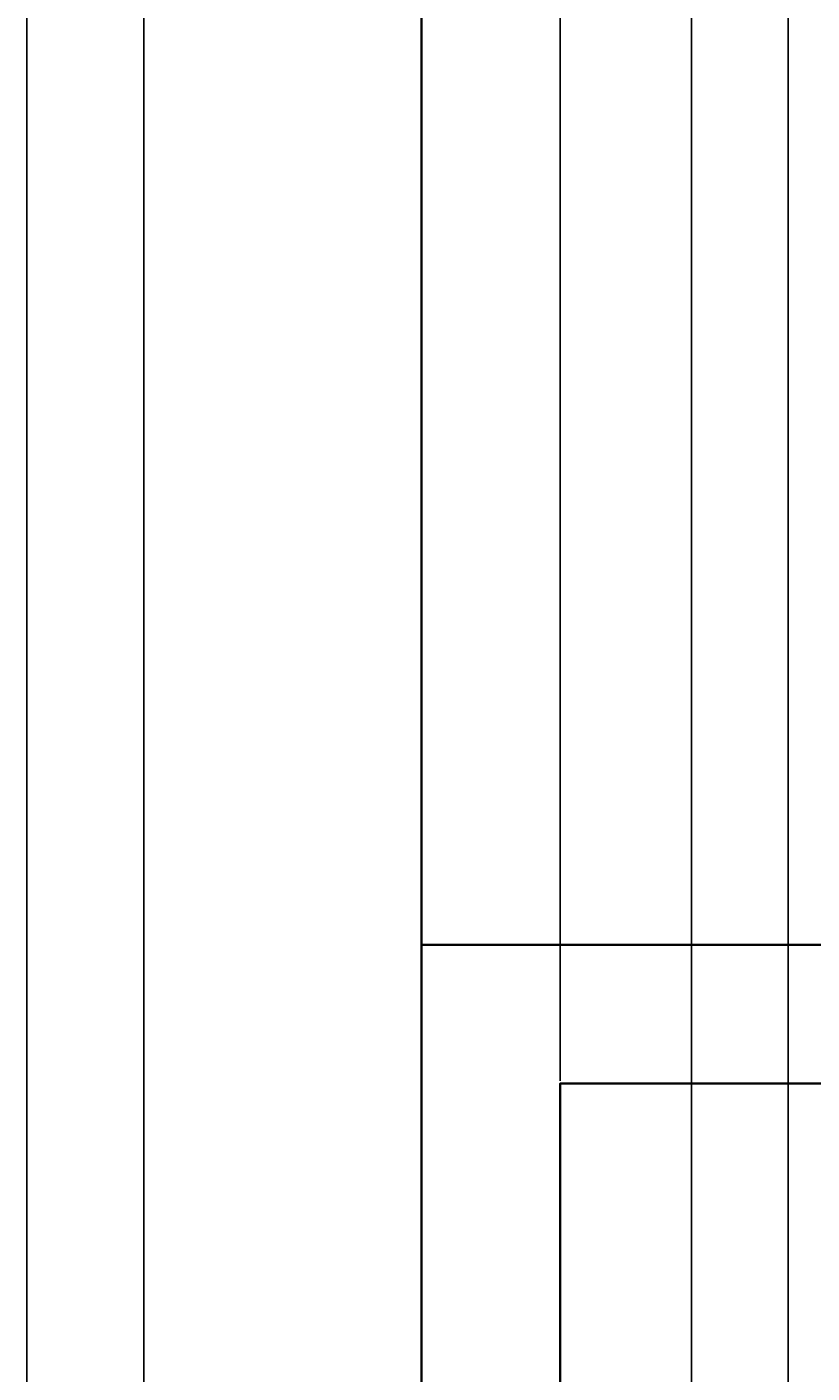
# Model space of a CAD drawing. Units: inches. Extents: x -6 to 289, y -8 to 323.
# Tile 50 of 107: x 107 to 124, y 153 to 182. Entities that reach past the tile are written whole.
import ezdxf

# ---------------------------------------------------------------- set-up
doc = ezdxf.new("R2010")
doc.units = ezdxf.units.IN
doc.header["$MEASUREMENT"] = 0
doc.layers.add('A-ANNO-DIMS', color=2, linetype='Continuous', lineweight=18)
doc.layers.add('A-ELEV', color=7, linetype='Continuous', lineweight=35)
doc.styles.get("Standard").update_dxf_attribs({"font": 'arial.ttf'})
doc.dimstyles.get("Standard").update_dxf_attribs({"dimtxt": 0.18, "dimasz": 0.18, "dimexe": 0.18, "dimexo": 0.0625, "dimgap": 0.09, "dimtad": 0, "dimtih": 1, "dimtoh": 1, "dimdec": 4, "dimzin": 0, "dimdsep": 46, "dimtxsty": 'Standard', "dimcen": 0.09, "dimadec": 0, "dimazin": 0, "dimtfac": 1, "dimtdec": 4, "dimtofl": 0, "dimtmove": 0, "dimatfit": 3, "dimfxl": 1, "dimtolj": 1, "dimtzin": 0, "dimarcsym": 0})

# ---------------------------------------------------------------- blocks, each defined once
blk = doc.blocks.new('*D58')
at = {"layer": 'A-ANNO-DIMS', "color": 0, "lineweight": -2, "transparency": 16777216}
for p, q in [((106.634, 68.495), (106.634, 322.969)), ((123.094, 68.495), (123.094, 322.969)), ((106.814, 322.789), (114.479, 322.789)), ((122.914, 322.789), (115.249, 322.789))]:
    blk.add_line(p, q, dxfattribs=at)
at = {"layer": 'A-ANNO-DIMS', "color": 0, "transparency": 16777216}
for points in [[(106.814, 322.819), (106.814, 322.759), (106.634, 322.789)], [(122.914, 322.819), (122.914, 322.759), (123.094, 322.789)]]:
    blk.add_solid(points, dxfattribs=at)
at = {"layer": 'Defpoints', "color": 0, "transparency": 16777216}
for p in [(123.094, 322.789), (106.634, 68.432), (123.094, 68.432)]:
    blk.add_point(p, dxfattribs=at)
at = {"layer": 'A-ANNO-DIMS', "color": 0, "transparency": 16777216, "insert": (114.864, 322.789), "char_height": 0.18, "attachment_point": 5}
blk.add_mtext('\\A1;16.46', dxfattribs=at)
blk = doc.blocks.new('*D73')
at = {"layer": 'A-ANNO-DIMS', "color": 0, "lineweight": -2, "transparency": 16777216}
for p, q in [((121.008, 51.148), (121.008, 322.969)), ((135.296, 51.148), (135.296, 322.969)), ((121.188, 322.789), (127.697, 322.789)), ((135.116, 322.789), (128.607, 322.789))]:
    blk.add_line(p, q, dxfattribs=at)
at = {"layer": 'A-ANNO-DIMS', "color": 0, "transparency": 16777216}
for points in [[(121.188, 322.819), (121.188, 322.759), (121.008, 322.789)], [(135.116, 322.819), (135.116, 322.759), (135.296, 322.789)]]:
    blk.add_solid(points, dxfattribs=at)
at = {"layer": 'Defpoints', "color": 0, "transparency": 16777216}
for p in [(135.296, 322.789), (121.008, 51.085), (135.296, 51.085)]:
    blk.add_point(p, dxfattribs=at)
at = {"layer": 'A-ANNO-DIMS', "color": 0, "transparency": 16777216, "insert": (128.152, 322.789), "char_height": 0.18, "attachment_point": 5}
blk.add_mtext('\\A1;14.288', dxfattribs=at)
blk = doc.blocks.new('*D92')
at = {"layer": 'A-ANNO-DIMS', "color": 0, "lineweight": -2, "transparency": 16777216}
for p, q in [((109.164, 127.351), (109.164, 322.969)), ((115.164, 162.411), (115.164, 322.969)), ((109.344, 322.789), (112.014, 322.789)), ((114.984, 322.789), (112.313, 322.789))]:
    blk.add_line(p, q, dxfattribs=at)
at = {"layer": 'A-ANNO-DIMS', "color": 0, "transparency": 16777216}
for points in [[(109.344, 322.819), (109.344, 322.759), (109.164, 322.789)], [(114.984, 322.819), (114.984, 322.759), (115.164, 322.789)]]:
    blk.add_solid(points, dxfattribs=at)
at = {"layer": 'Defpoints', "color": 0, "transparency": 16777216}
for p in [(115.164, 322.789), (115.164, 162.348), (109.164, 127.289)]:
    blk.add_point(p, dxfattribs=at)
at = {"layer": 'A-ANNO-DIMS', "color": 0, "transparency": 16777216, "insert": (112.164, 322.789), "char_height": 0.18, "attachment_point": 5}
blk.add_mtext('\\A1;6', dxfattribs=at)
blk = doc.blocks.new('*D93')
at = {"layer": 'A-ANNO-DIMS', "color": 0, "lineweight": -2, "transparency": 16777216}
for p, q in [((115.164, 162.411), (115.164, 322.969)), ((118.164, 159.411), (118.164, 322.969)), ((115.344, 322.789), (116.515, 322.789)), ((117.984, 322.789), (116.813, 322.789))]:
    blk.add_line(p, q, dxfattribs=at)
at = {"layer": 'A-ANNO-DIMS', "color": 0, "transparency": 16777216}
for points in [[(115.344, 322.819), (115.344, 322.759), (115.164, 322.789)], [(117.984, 322.819), (117.984, 322.759), (118.164, 322.789)]]:
    blk.add_solid(points, dxfattribs=at)
at = {"layer": 'Defpoints', "color": 0, "transparency": 16777216}
for p in [(118.164, 322.789), (115.164, 162.348), (118.164, 159.348)]:
    blk.add_point(p, dxfattribs=at)
at = {"layer": 'A-ANNO-DIMS', "color": 0, "transparency": 16777216, "insert": (116.664, 322.789), "char_height": 0.18, "attachment_point": 5}
blk.add_mtext('\\A1;3', dxfattribs=at)
blk = doc.blocks.new('*D94')
at = {"layer": 'A-ANNO-DIMS', "color": 0, "lineweight": -2, "transparency": 16777216}
for p, q in [((118.164, 159.411), (118.164, 322.969)), ((161.552, 159.411), (161.552, 322.969)), ((118.344, 322.789), (139.46, 322.789)), ((161.372, 322.789), (140.256, 322.789))]:
    blk.add_line(p, q, dxfattribs=at)
at = {"layer": 'A-ANNO-DIMS', "color": 0, "transparency": 16777216}
for points in [[(118.344, 322.819), (118.344, 322.759), (118.164, 322.789)], [(161.372, 322.819), (161.372, 322.759), (161.552, 322.789)]]:
    blk.add_solid(points, dxfattribs=at)
at = {"layer": 'Defpoints', "color": 0, "transparency": 16777216}
for p in [(161.552, 322.789), (118.164, 159.348), (161.552, 159.348)]:
    blk.add_point(p, dxfattribs=at)
at = {"layer": 'A-ANNO-DIMS', "color": 0, "transparency": 16777216, "insert": (139.858, 322.789), "char_height": 0.18, "attachment_point": 5}
blk.add_mtext('\\A1;43.39', dxfattribs=at)

msp = doc.modelspace()

# ---------------------------------------------------------------- linework, layer by layer
at = {"layer": 'A-ELEV'}
msp.add_line((115.1638, 247.2888), (115.1638, 139.2888), dxfattribs=at)
for points in [[(247.1638, 139.2888), (115.1638, 139.2888), (115.1638, 162.3484), (247.1638, 162.3484)], [(244.1638, 142.2888), (118.1638, 142.2888), (118.1638, 159.3484), (244.1638, 159.3484)]]:
    msp.add_lwpolyline(points, close=True, dxfattribs=at)

# ---------------------------------------------------------------- dimensions: what is measured, and where the dimension line sits
at = {"layer": 'A-ANNO-DIMS'}
for base, p1, p2, override, picture, middle in [((123.094, 322.7888), (106.634, 68.4322), (123.094, 68.4322), {"dimdec": 2, "dimlfac": 1, "dimrnd": 0, "dimzin": 0, "dimdsep": 46, "dimlunit": 2}, '*D58', (114.864, 322.7888)), ((115.1638, 322.7888), (109.1638, 127.2888), (115.1638, 162.3484), {"dimdec": 0, "dimlfac": 1, "dimrnd": 0, "dimzin": 0, "dimdsep": 46, "dimlunit": 2}, '*D92', (112.1638, 322.7888)), ((118.1638, 322.7888), (115.1638, 162.3484), (118.1638, 159.3484), {"dimdec": 0, "dimlfac": 1, "dimrnd": 0, "dimzin": 0, "dimdsep": 46, "dimlunit": 2}, '*D93', (116.6638, 322.7888)), ((161.5522, 322.7888), (118.1638, 159.3484), (161.5522, 159.3484), {"dimdec": 2, "dimlfac": 1, "dimrnd": 0, "dimzin": 0, "dimdsep": 46, "dimlunit": 2}, '*D94', (139.858, 322.7888)), ((135.296, 322.7888), (121.008, 51.0851), (135.296, 51.0851), {"dimdec": 3, "dimlfac": 1, "dimrnd": 0, "dimzin": 0, "dimdsep": 46, "dimlunit": 2}, '*D73', (128.152, 322.7888))]:
    dim = msp.add_linear_dim(base=base, p1=p1, p2=p2, dimstyle='Standard', override=override, dxfattribs=at)
    dim.commit()
    dim.dimension.update_dxf_attribs({"geometry": picture, "text_midpoint": middle})

doc.saveas('drawing.dxf')
